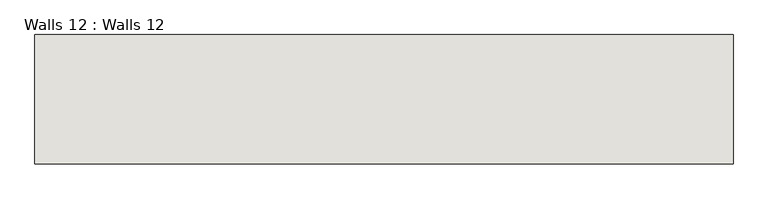
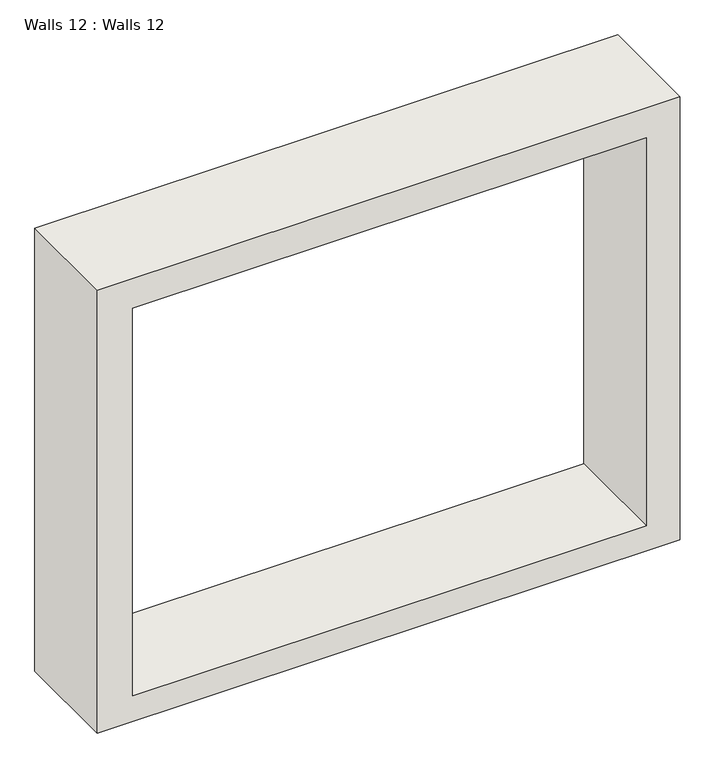
"""IFC4 building model written with IfcOpenShell, lengths in millimetres: wall geometry, Walls 12 : Walls 12."""

from ifc_helpers import new_model, si_unit, frame, origin, place, context, project, spatial, polyline, outline, extrude, source, transform, mapped, element, save


def walls_12_walls_12_7f8ca245(model_context):
    return source(origin(), model_context, "Body", "SweptSolid", [
        extrude(outline(polyline([(3917.8465326, -9558.0907032), (3917.8465326, -7913.8407032), (5238.75, -7913.8407032), (5238.75, -9558.0907032), (3917.8465326, -9558.0907032)]), holes=[polyline([(3994.15, -9457.5560427), (5149.85, -9457.5560427), (5149.85, -8008.6907032), (3994.15, -8008.6907032), (3994.15, -9457.5560427)])]), frame((0.0, 3537.1456099, 0.0), z_axis=(0.0, 1.0, 0.0), x_axis=(0.0, 0.0, 1.0)), (0.0, 0.0, 1.0), 304.8),
    ])


if __name__ == "__main__":
    model = new_model("IFC4")
    model_context = context("Model", 3, world=origin())
    ifc_project = project(units=[si_unit("LENGTHUNIT", "METRE", prefix="MILLI")], contexts=[model_context])
    site = spatial("IfcSite", under=ifc_project)
    building = spatial("IfcBuilding", under=site)
    placement = place(None, origin())
    walls_12_walls_12_shape = walls_12_walls_12_7f8ca245(model_context)
    element("IfcWall", 1, ObjectType="Walls 12 : Walls 12", at=placement, inside=building, context=model_context, shape_type="MappedRepresentation", body=[
        mapped(walls_12_walls_12_shape, transform((0.0, 0.0, 0.0), x_axis=(1.0, 0.0, 0.0), y_axis=(0.0, 1.0, 0.0), z_axis=(0.0, 0.0, 1.0))),
    ])
    save(model, "model.ifc")

# Revit data of these elements
# Element 1 (IfcWall, "Walls 12 : Walls 12")
#   Materials on its faces: "Default Wall"
# Materials
#   "Default Wall": colour RGB 80 80 80, transparency 0
